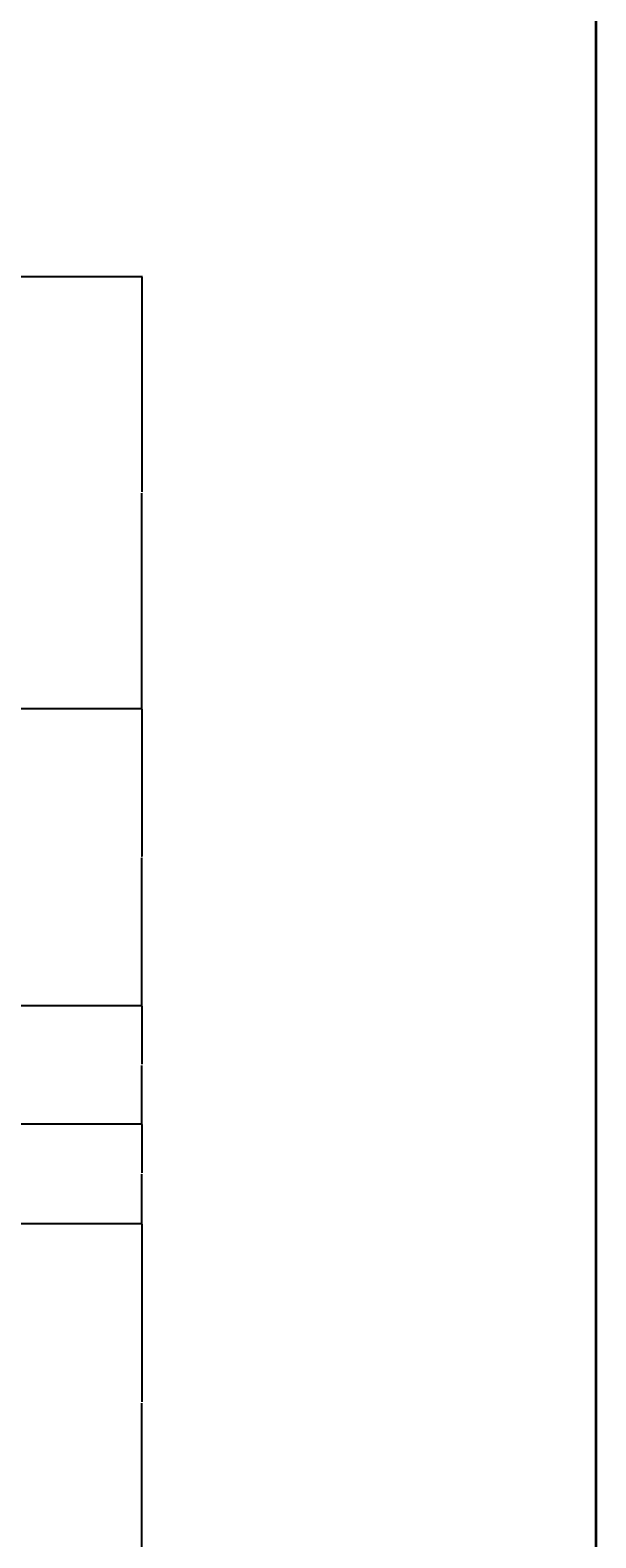
# Model space of a CAD drawing. Units: inches. Extents: x 2165 to 3042, y 1626 to 2968.
# Tile 10 of 11: x 2889 to 3042, y 1990 to 2399. Entities that reach past the tile are written whole.
import ezdxf

# ---------------------------------------------------------------- set-up
doc = ezdxf.new("R2010")
doc.units = ezdxf.units.IN
doc.layers.add('A-ANNO-DIMS', color=2, linetype='Continuous', lineweight=18)
doc.layers.add('A-WALL', color=7, linetype='Continuous', lineweight=35)
doc.styles.get("Standard").update_dxf_attribs({"font": 'arial.ttf'})
doc.dimstyles.get("Standard").update_dxf_attribs({"dimtxt": 0.18, "dimasz": 0.18, "dimexe": 0.18, "dimexo": 0.0625, "dimgap": 0.09, "dimtad": 0, "dimtih": 1, "dimtoh": 1, "dimdec": 4, "dimzin": 0, "dimdsep": 46, "dimtxsty": 'Standard', "dimcen": 0.09, "dimadec": 0, "dimazin": 0, "dimtfac": 1, "dimtdec": 4, "dimtofl": 0, "dimtmove": 0, "dimatfit": 3, "dimfxl": 1, "dimtolj": 1, "dimtzin": 0, "dimarcsym": 0})

# ---------------------------------------------------------------- blocks, each defined once
blk = doc.blocks.new('*D58')
at = {"layer": 'A-ANNO-DIMS', "color": 0, "lineweight": -2, "transparency": 16777216}
for p, q in [((2885.17, 2075.58), (2919.58, 2075.58)), ((2919.4, 2075.4), (2919.4, 2027.26)), ((2919.4, 1978.76), (2919.4, 2026.9)), ((2880.67, 1978.58), (2919.58, 1978.58))]:
    blk.add_line(p, q, dxfattribs=at)
at = {"layer": 'A-ANNO-DIMS', "color": 0, "transparency": 16777216}
for points in [[(2919.37, 2075.4), (2919.43, 2075.4), (2919.4, 2075.58)], [(2919.37, 1978.76), (2919.43, 1978.76), (2919.4, 1978.58)]]:
    blk.add_solid(points, dxfattribs=at)
at = {"layer": 'Defpoints', "color": 0, "transparency": 16777216}
for p in [(2885.1, 2075.58), (2919.4, 2075.58), (2880.6, 1978.58)]:
    blk.add_point(p, dxfattribs=at)
at = {"layer": 'A-ANNO-DIMS', "color": 0, "transparency": 16777216, "insert": (2919.4, 2027.08), "char_height": 0.18, "attachment_point": 5}
blk.add_mtext('\\A1;97', dxfattribs=at)
blk = doc.blocks.new('*D59')
at = {"layer": 'A-ANNO-DIMS', "color": 0, "lineweight": -2, "transparency": 16777216}
for p, q in [((2829.92, 2102.58), (2919.58, 2102.58)), ((2919.4, 2102.4), (2919.4, 2089.26)), ((2919.4, 2075.76), (2919.4, 2088.9)), ((2885.17, 2075.58), (2919.58, 2075.58))]:
    blk.add_line(p, q, dxfattribs=at)
at = {"layer": 'A-ANNO-DIMS', "color": 0, "transparency": 16777216}
for points in [[(2919.37, 2102.4), (2919.43, 2102.4), (2919.4, 2102.58)], [(2919.37, 2075.76), (2919.43, 2075.76), (2919.4, 2075.58)]]:
    blk.add_solid(points, dxfattribs=at)
at = {"layer": 'Defpoints', "color": 0, "transparency": 16777216}
for p in [(2829.85, 2102.58), (2919.4, 2102.58), (2885.1, 2075.58)]:
    blk.add_point(p, dxfattribs=at)
at = {"layer": 'A-ANNO-DIMS', "color": 0, "transparency": 16777216, "insert": (2919.4, 2089.08), "char_height": 0.18, "attachment_point": 5}
blk.add_mtext('\\A1;27', dxfattribs=at)
blk = doc.blocks.new('*D60')
at = {"layer": 'A-ANNO-DIMS', "color": 0, "lineweight": -2, "transparency": 16777216}
for p, q in [((2885.17, 2134.58), (2919.58, 2134.58)), ((2919.4, 2134.4), (2919.4, 2118.76)), ((2919.4, 2102.76), (2919.4, 2118.4)), ((2829.92, 2102.58), (2919.58, 2102.58))]:
    blk.add_line(p, q, dxfattribs=at)
at = {"layer": 'A-ANNO-DIMS', "color": 0, "transparency": 16777216}
for points in [[(2919.37, 2134.4), (2919.43, 2134.4), (2919.4, 2134.58)], [(2919.37, 2102.76), (2919.43, 2102.76), (2919.4, 2102.58)]]:
    blk.add_solid(points, dxfattribs=at)
at = {"layer": 'Defpoints', "color": 0, "transparency": 16777216}
for p in [(2885.1, 2134.58), (2919.4, 2134.58), (2829.85, 2102.58)]:
    blk.add_point(p, dxfattribs=at)
at = {"layer": 'A-ANNO-DIMS', "color": 0, "transparency": 16777216, "insert": (2919.4, 2118.58), "char_height": 0.18, "attachment_point": 5}
blk.add_mtext('\\A1;32', dxfattribs=at)
blk = doc.blocks.new('*D61')
at = {"layer": 'A-ANNO-DIMS', "color": 0, "lineweight": -2, "transparency": 16777216}
for p, q in [((2880.67, 2215.08), (2919.58, 2215.08)), ((2919.4, 2214.9), (2919.4, 2175.01)), ((2919.4, 2134.76), (2919.4, 2174.65)), ((2885.17, 2134.58), (2919.58, 2134.58))]:
    blk.add_line(p, q, dxfattribs=at)
at = {"layer": 'A-ANNO-DIMS', "color": 0, "transparency": 16777216}
for points in [[(2919.37, 2214.9), (2919.43, 2214.9), (2919.4, 2215.08)], [(2919.37, 2134.76), (2919.43, 2134.76), (2919.4, 2134.58)]]:
    blk.add_solid(points, dxfattribs=at)
at = {"layer": 'Defpoints', "color": 0, "transparency": 16777216}
for p in [(2880.6, 2215.08), (2919.4, 2215.08), (2885.1, 2134.58)]:
    blk.add_point(p, dxfattribs=at)
at = {"layer": 'A-ANNO-DIMS', "color": 0, "transparency": 16777216, "insert": (2919.4, 2174.83), "char_height": 0.18, "attachment_point": 5}
blk.add_mtext('\\A1;80.5', dxfattribs=at)
blk = doc.blocks.new('*D62')
at = {"layer": 'A-ANNO-DIMS', "color": 0, "lineweight": -2, "transparency": 16777216}
for p, q in [((2885.17, 2332.08), (2919.58, 2332.08)), ((2919.4, 2331.9), (2919.4, 2273.76)), ((2919.4, 2215.26), (2919.4, 2273.4)), ((2880.67, 2215.08), (2919.58, 2215.08))]:
    blk.add_line(p, q, dxfattribs=at)
at = {"layer": 'A-ANNO-DIMS', "color": 0, "transparency": 16777216}
for points in [[(2919.37, 2331.9), (2919.43, 2331.9), (2919.4, 2332.08)], [(2919.37, 2215.26), (2919.43, 2215.26), (2919.4, 2215.08)]]:
    blk.add_solid(points, dxfattribs=at)
at = {"layer": 'Defpoints', "color": 0, "transparency": 16777216}
for p in [(2885.1, 2332.08), (2919.4, 2332.08), (2880.6, 2215.08)]:
    blk.add_point(p, dxfattribs=at)
at = {"layer": 'A-ANNO-DIMS', "color": 0, "transparency": 16777216, "insert": (2919.4, 2273.58), "char_height": 0.18, "attachment_point": 5}
blk.add_mtext('\\A1;117', dxfattribs=at)

msp = doc.modelspace()

# ---------------------------------------------------------------- linework, layer by layer
at = {"layer": 'A-WALL'}
msp.add_lwpolyline([(2191.9961, 2967.8547), (3042.3708, 2967.8547), (3042.3708, 1626.3264), (2191.9961, 1626.3264)], close=True, dxfattribs=at)

# ---------------------------------------------------------------- dimensions: what is measured, and where the dimension line sits
at = {"layer": 'A-ANNO-DIMS'}
for base, p1, p2, override, picture, middle in [((2919.4045, 2332.0783), (2880.6045, 2215.0783), (2885.1045, 2332.0783), {"dimdec": 0, "dimlfac": 1, "dimrnd": 0, "dimzin": 0, "dimdsep": 46, "dimlunit": 2}, '*D62', (2919.4045, 2273.5783)), ((2919.4045, 2215.0783), (2885.1045, 2134.5783), (2880.6045, 2215.0783), {"dimdec": 1, "dimlfac": 1, "dimrnd": 0, "dimzin": 0, "dimdsep": 46, "dimlunit": 2}, '*D61', (2919.4045, 2174.8283)), ((2919.4045, 2134.5783), (2829.8545, 2102.5783), (2885.1045, 2134.5783), {"dimdec": 0, "dimlfac": 1, "dimrnd": 0, "dimzin": 0, "dimdsep": 46, "dimlunit": 2}, '*D60', (2919.4045, 2118.5783)), ((2919.4045, 2102.5783), (2885.1045, 2075.5783), (2829.8545, 2102.5783), {"dimdec": 0, "dimlfac": 1, "dimrnd": 0, "dimzin": 0, "dimdsep": 46, "dimlunit": 2}, '*D59', (2919.4045, 2089.0783)), ((2919.4045, 2075.5783), (2880.6045, 1978.5783), (2885.1045, 2075.5783), {"dimdec": 0, "dimlfac": 1, "dimrnd": 0, "dimzin": 0, "dimdsep": 46, "dimlunit": 2}, '*D58', (2919.4045, 2027.0783))]:
    dim = msp.add_linear_dim(base=base, p1=p1, p2=p2, angle=90, dimstyle='Standard', override=override, dxfattribs=at)
    dim.commit()
    dim.dimension.update_dxf_attribs({"geometry": picture, "text_midpoint": middle})

doc.saveas('drawing.dxf')
